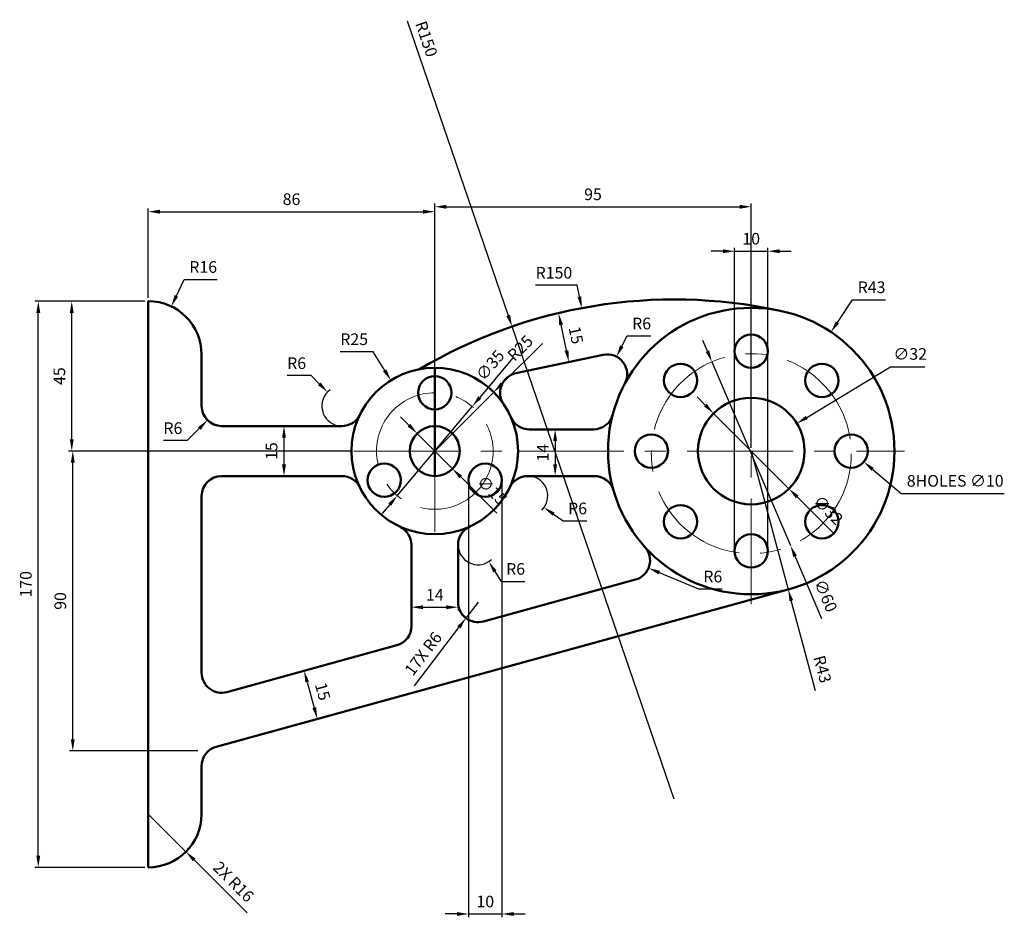
# Model space of a CAD drawing. Units: millimetres. Extents: x -39 to 257, y -15 to 255.
import ezdxf

# ---------------------------------------------------------------- set-up
doc = ezdxf.new("R2010")
doc.units = ezdxf.units.MM
doc.linetypes.add('CENTER', pattern=[50.8, 31.75, -6.35, 6.35, -6.35])
for name, color, linetype, lineweight in [('M-CNTR', 4, 'CENTER', 18), ('M-CONS', 8, 'Continuous', 13), ('M-DIMS', 3, 'Continuous', 25), ('M-OUTL', 7, 'Continuous', 50)]:
    doc.layers.add(name, color=color, linetype=linetype, lineweight=lineweight)
doc.styles.get("Standard").update_dxf_attribs({"font": 'arial.ttf'})
doc.dimstyles.new('AM_ISO$0', dxfattribs={"dimtxt": 3.5, "dimasz": 3.5, "dimexe": 1, "dimexo": 1, "dimgap": 1.5, "dimtad": 1, "dimdsep": 46, "dimtxsty": 'Standard', "dimcen": 0, "dimclrd": 256, "dimclre": 256, "dimclrt": 2, "dimadec": 0, "dimazin": 2, "dimtp": 0.1, "dimtm": 0.1, "dimtfac": 0.71, "dimtdec": 3, "dimtmove": 0, "dimatfit": 3, "dimfxl": 1, "dimlwd": -1, "dimlwe": -1, "dimarcsym": 1})
doc.dimstyles.new('AM_ISO$3', dxfattribs={"dimtxt": 3.5, "dimasz": 3.5, "dimexe": 1, "dimexo": 1, "dimgap": 1.5, "dimtad": 1, "dimtoh": 1, "dimdsep": 46, "dimtxsty": 'Standard', "dimcen": 0, "dimclrd": 256, "dimclre": 256, "dimclrt": 2, "dimadec": 0, "dimazin": 2, "dimtp": 0.1, "dimtm": 0.1, "dimtfac": 0.71, "dimtdec": 3, "dimtofl": 0, "dimtmove": 0, "dimatfit": 0, "dimfxl": 1, "dimlwd": -1, "dimlwe": -1, "dimarcsym": 1})
doc.dimstyles.new('AM_ISO$4', dxfattribs={"dimtxt": 3.5, "dimasz": 3.5, "dimexe": 1, "dimexo": 1, "dimgap": 1.5, "dimtad": 1, "dimtoh": 1, "dimdsep": 46, "dimtxsty": 'Standard', "dimcen": 0, "dimclrd": 256, "dimclre": 256, "dimclrt": 2, "dimadec": 0, "dimazin": 2, "dimtp": 0.1, "dimtm": 0.1, "dimtfac": 0.71, "dimtdec": 3, "dimtofl": 0, "dimtmove": 0, "dimatfit": 0, "dimfxl": 1, "dimlwd": -1, "dimlwe": -1, "dimarcsym": 1})

# ---------------------------------------------------------------- blocks, each defined once
blk = doc.blocks.new('*D3')
at = {"layer": 'Defpoints', "color": 0, "transparency": 16777216}
for p in [(-33.02, 170), (0, 170), (0, 0)]:
    blk.add_point(p, dxfattribs=at)
at = {"layer": 'M-DIMS', "color": 0, "linetype": 'ByBlock', "transparency": 16777216}
for p, q in [((-1, 170), (-34.02, 170)), ((-33.02, 3.5), (-33.02, 166.5)), ((-1, 0), (-34.02, 0))]:
    blk.add_line(p, q, dxfattribs=at)
at = {"layer": 'M-DIMS', "color": 0, "transparency": 16777216}
for points in [[(-33.61, 166.5), (-32.44, 166.5), (-33.02, 170)], [(-33.61, 3.5), (-32.44, 3.5), (-33.02, 0)]]:
    blk.add_solid(points, dxfattribs=at)
at = {"layer": 'M-DIMS', "color": 0, "transparency": 16777216, "insert": (-36.31, 85), "char_height": 3.5, "attachment_point": 5, "rotation": 90}
blk.add_mtext('170', dxfattribs=at)
blk = doc.blocks.new('*U4')
blk.add_circle((0, 0), 5)
blk = doc.blocks.new('*U5')
at = {"layer": 'M-OUTL', "color": 0, "linetype": 'ByBlock', "lineweight": -2, "transparency": 16777216}
for p, rotation in [((181, 154.99), 90), ((159.79, 146.21), 135), ((202.21, 146.21), 45), ((151.01, 125), 180), ((159.79, 103.79), 225), ((202.21, 103.79), 315), ((181, 95.01), 270)]:
    blk.add_blockref('*U4', p, dxfattribs=dict(at, rotation=rotation))
blk.add_blockref('*U4', (210.99, 125), dxfattribs=at)
blk = doc.blocks.new('*U6')
blk.add_circle((0, 0), 5)
blk = doc.blocks.new('*U7')
at = {"layer": 'M-OUTL', "color": 0, "linetype": 'ByBlock', "lineweight": -2, "transparency": 16777216}
blk.add_blockref('*U6', (86, 142.5), dxfattribs=at)
for p, rotation in [((70.84, 116.25), 120), ((101.16, 116.25), 240)]:
    blk.add_blockref('*U6', p, dxfattribs=dict(at, rotation=rotation))
blk = doc.blocks.new('*D8')
at = {"layer": 'Defpoints', "color": 0, "transparency": 16777216}
for p in [(144.62, 92.17), (150.16, 89.85)]:
    blk.add_point(p, dxfattribs=at)
at = {"layer": 'M-DIMS', "color": 0, "linetype": 'ByBlock', "transparency": 16777216}
for p, q in [((153.38, 88.5), (165.14, 83.58)), ((165.14, 83.58), (172.28, 83.58))]:
    blk.add_line(p, q, dxfattribs=at)
at = {"layer": 'M-DIMS', "color": 0, "transparency": 16777216}
blk.add_solid([(153.61, 89.04), (153.16, 87.96), (150.16, 89.85)], dxfattribs=at)
at = {"layer": 'M-DIMS', "color": 0, "transparency": 16777216, "insert": (169.46, 86.86), "char_height": 3.5, "attachment_point": 5}
blk.add_mtext('R6', dxfattribs=at)
blk = doc.blocks.new('*D9')
at = {"layer": 'Defpoints', "color": 0, "transparency": 16777216}
for p in [(99, 96.86), (102.2, 91.78)]:
    blk.add_point(p, dxfattribs=at)
at = {"layer": 'M-DIMS', "color": 0, "linetype": 'ByBlock', "transparency": 16777216}
for p, q in [((104.07, 88.83), (105.94, 85.87)), ((105.94, 85.87), (113.08, 85.87))]:
    blk.add_line(p, q, dxfattribs=at)
blk.add_arc((99, 96.86), 6, 189.5493, 311.8304, dxfattribs=at)
at = {"layer": 'M-DIMS', "color": 0, "transparency": 16777216}
blk.add_solid([(104.57, 89.14), (103.58, 88.51), (102.2, 91.78)], dxfattribs=at)
at = {"layer": 'M-DIMS', "color": 0, "transparency": 16777216, "insert": (110.26, 89.15), "char_height": 3.5, "attachment_point": 5}
blk.add_mtext('R6', dxfattribs=at)
blk = doc.blocks.new('*D10')
at = {"layer": 'Defpoints', "color": 0, "transparency": 16777216}
for p in [(22, 138.5), (17.77, 134.25)]:
    blk.add_point(p, dxfattribs=at)
at = {"layer": 'M-DIMS', "color": 0, "linetype": 'ByBlock', "transparency": 16777216}
for p, q in [((15.3, 131.76), (11.7, 128.14)), ((11.7, 128.14), (4.56, 128.14))]:
    blk.add_line(p, q, dxfattribs=at)
at = {"layer": 'M-DIMS', "color": 0, "transparency": 16777216}
blk.add_solid([(14.89, 132.17), (15.72, 131.35), (17.77, 134.25)], dxfattribs=at)
at = {"layer": 'M-DIMS', "color": 0, "transparency": 16777216, "insert": (7.38, 131.42), "char_height": 3.5, "attachment_point": 5}
blk.add_mtext('R6', dxfattribs=at)
blk = doc.blocks.new('*D11')
at = {"layer": 'Defpoints', "color": 0, "transparency": 16777216}
for p in [(86, 196.87), (0, 170), (86, 125)]:
    blk.add_point(p, dxfattribs=at)
at = {"layer": 'M-DIMS', "color": 0, "linetype": 'ByBlock', "transparency": 16777216}
for p, q in [((0, 171), (0, 197.87)), ((3.5, 196.87), (82.5, 196.87)), ((86, 126), (86, 197.87))]:
    blk.add_line(p, q, dxfattribs=at)
at = {"layer": 'M-DIMS', "color": 0, "transparency": 16777216}
for points in [[(3.5, 197.45), (3.5, 196.28), (0, 196.87)], [(82.5, 197.45), (82.5, 196.28), (86, 196.87)]]:
    blk.add_solid(points, dxfattribs=at)
at = {"layer": 'M-DIMS', "color": 0, "transparency": 16777216, "insert": (43, 200.16), "char_height": 3.5, "attachment_point": 5}
blk.add_mtext('86', dxfattribs=at)
blk = doc.blocks.new('*D12')
at = {"layer": 'Defpoints', "color": 0, "transparency": 16777216}
for p in [(181, 198.35), (86, 125), (181, 125)]:
    blk.add_point(p, dxfattribs=at)
at = {"layer": 'M-DIMS', "color": 0, "linetype": 'ByBlock', "transparency": 16777216}
for p, q in [((86, 126), (86, 199.35)), ((89.5, 198.35), (177.5, 198.35)), ((181, 126), (181, 199.35))]:
    blk.add_line(p, q, dxfattribs=at)
at = {"layer": 'M-DIMS', "color": 0, "transparency": 16777216}
for points in [[(89.5, 198.93), (89.5, 197.76), (86, 198.35)], [(177.5, 198.93), (177.5, 197.76), (181, 198.35)]]:
    blk.add_solid(points, dxfattribs=at)
at = {"layer": 'M-DIMS', "color": 0, "transparency": 16777216, "insert": (133.5, 201.63), "char_height": 3.5, "attachment_point": 5}
blk.add_mtext('95', dxfattribs=at)
blk = doc.blocks.new('*D13')
at = {"layer": 'Defpoints', "color": 0, "transparency": 16777216}
for p in [(6.91, 168.43), (0, 154)]:
    blk.add_point(p, dxfattribs=at)
at = {"layer": 'M-DIMS', "color": 0, "linetype": 'ByBlock', "transparency": 16777216}
for p, q in [((8.43, 171.59), (10.79, 176.52)), ((10.79, 176.52), (20.65, 176.52))]:
    blk.add_line(p, q, dxfattribs=at)
at = {"layer": 'M-DIMS', "color": 0, "transparency": 16777216}
blk.add_solid([(7.9, 171.84), (8.95, 171.33), (6.91, 168.43)], dxfattribs=at)
at = {"layer": 'M-DIMS', "color": 0, "transparency": 16777216, "insert": (16.47, 179.81), "char_height": 3.5, "attachment_point": 5}
blk.add_mtext('R16', dxfattribs=at)
blk = doc.blocks.new('*D14')
at = {"layer": 'Defpoints', "color": 0, "transparency": 16777216}
for p in [(49.09, 59.66), (50.75, 44.56), (53.07, 45.2)]:
    blk.add_point(p, dxfattribs=at)
at = {"layer": 'M-DIMS', "color": 0, "linetype": 'ByBlock', "transparency": 16777216}
for p, q in [((48.13, 59.4), (45.81, 58.76)), ((47.7, 55.65), (49.82, 47.94)), ((52.11, 44.94), (49.79, 44.3))]:
    blk.add_line(p, q, dxfattribs=at)
at = {"layer": 'M-DIMS', "color": 0, "transparency": 16777216}
for points in [[(48.26, 55.81), (47.14, 55.5), (46.77, 59.02)], [(50.39, 48.09), (49.26, 47.78), (50.75, 44.56)]]:
    blk.add_solid(points, dxfattribs=at)
at = {"layer": 'M-DIMS', "color": 0, "transparency": 16777216, "insert": (51.93, 52.67), "char_height": 3.5, "attachment_point": 5, "rotation": 285.3849}
blk.add_mtext('15', dxfattribs=at)
blk = doc.blocks.new('*D15')
at = {"layer": 'Defpoints', "color": 0, "transparency": 16777216}
for p in [(79, 84.66), (93, 84.66), (93, 78.11)]:
    blk.add_point(p, dxfattribs=at)
at = {"layer": 'M-DIMS', "color": 0, "linetype": 'ByBlock', "transparency": 16777216}
for p, q in [((79, 83.66), (79, 77.11)), ((93, 83.66), (93, 77.11)), ((82.5, 78.11), (89.5, 78.11))]:
    blk.add_line(p, q, dxfattribs=at)
at = {"layer": 'M-DIMS', "color": 0, "transparency": 16777216}
for points in [[(82.5, 78.69), (82.5, 77.52), (79, 78.11)], [(89.5, 78.69), (89.5, 77.52), (93, 78.11)]]:
    blk.add_solid(points, dxfattribs=at)
at = {"layer": 'M-DIMS', "color": 0, "transparency": 16777216, "insert": (86, 81.36), "char_height": 3.5, "attachment_point": 5}
blk.add_mtext('14', dxfattribs=at)
blk = doc.blocks.new('*D16')
at = {"layer": 'Defpoints', "color": 0, "transparency": 16777216}
for p in [(40.05, 132.5), (40.74, 132.5), (40.05, 117.5)]:
    blk.add_point(p, dxfattribs=at)
at = {"layer": 'M-DIMS', "color": 0, "linetype": 'ByBlock', "transparency": 16777216}
for p, q in [((41.05, 132.5), (41.74, 132.5)), ((40.74, 121), (40.74, 129)), ((41.05, 117.5), (41.74, 117.5))]:
    blk.add_line(p, q, dxfattribs=at)
at = {"layer": 'M-DIMS', "color": 0, "transparency": 16777216}
for points in [[(40.15, 129), (41.32, 129), (40.74, 132.5)], [(40.15, 121), (41.32, 121), (40.74, 117.5)]]:
    blk.add_solid(points, dxfattribs=at)
at = {"layer": 'M-DIMS', "color": 0, "transparency": 16777216, "insert": (37.45, 125), "char_height": 3.5, "attachment_point": 5, "rotation": 90}
blk.add_mtext('15', dxfattribs=at)
blk = doc.blocks.new('*D17')
at = {"layer": 'Defpoints', "color": 0, "transparency": 16777216}
for p in [(-22.67, 125), (62.15, 125), (15.85, 34.96)]:
    blk.add_point(p, dxfattribs=at)
at = {"layer": 'M-DIMS', "color": 0, "linetype": 'ByBlock', "transparency": 16777216}
for p, q in [((61.15, 125), (-23.67, 125)), ((-22.67, 38.46), (-22.67, 121.5)), ((14.85, 34.96), (-23.67, 34.96))]:
    blk.add_line(p, q, dxfattribs=at)
at = {"layer": 'M-DIMS', "color": 0, "transparency": 16777216}
for points in [[(-23.26, 121.5), (-22.09, 121.5), (-22.67, 125)], [(-23.26, 38.46), (-22.09, 38.46), (-22.67, 34.96)]]:
    blk.add_solid(points, dxfattribs=at)
at = {"layer": 'M-DIMS', "color": 0, "transparency": 16777216, "insert": (-25.96, 79.98), "char_height": 3.5, "attachment_point": 5, "rotation": 90}
blk.add_mtext('90', dxfattribs=at)
blk = doc.blocks.new('*D18')
at = {"layer": 'Defpoints', "color": 0, "transparency": 16777216}
for p in [(-22.97, 170), (0, 170), (61, 125)]:
    blk.add_point(p, dxfattribs=at)
at = {"layer": 'M-DIMS', "color": 0, "linetype": 'ByBlock', "transparency": 16777216}
for p, q in [((-1, 170), (-23.97, 170)), ((-22.97, 128.5), (-22.97, 166.5)), ((60, 125), (-23.97, 125))]:
    blk.add_line(p, q, dxfattribs=at)
at = {"layer": 'M-DIMS', "color": 0, "transparency": 16777216}
for points in [[(-23.56, 166.5), (-22.39, 166.5), (-22.97, 170)], [(-23.56, 128.5), (-22.39, 128.5), (-22.97, 125)]]:
    blk.add_solid(points, dxfattribs=at)
at = {"layer": 'M-DIMS', "color": 0, "transparency": 16777216, "insert": (-26.25, 147.5), "char_height": 3.5, "attachment_point": 5, "rotation": 90}
blk.add_mtext('45', dxfattribs=at)
blk = doc.blocks.new('*D19')
at = {"layer": 'Defpoints', "color": 0, "transparency": 16777216}
for p in [(53.83, 142.72), (58.09, 138.5)]:
    blk.add_point(p, dxfattribs=at)
at = {"layer": 'M-DIMS', "color": 0, "linetype": 'ByBlock', "transparency": 16777216}
for p, q in [((48.85, 147.64), (41.71, 147.64)), ((51.34, 145.18), (48.85, 147.64))]:
    blk.add_line(p, q, dxfattribs=at)
blk.add_arc((58.09, 138.5), 6, 125.7636, 260.4507, dxfattribs=at)
at = {"layer": 'M-DIMS', "color": 0, "transparency": 16777216}
blk.add_solid([(51.75, 145.6), (50.93, 144.77), (53.83, 142.72)], dxfattribs=at)
at = {"layer": 'M-DIMS', "color": 0, "transparency": 16777216, "insert": (44.53, 150.93), "char_height": 3.5, "attachment_point": 5}
blk.add_mtext('R6', dxfattribs=at)
blk = doc.blocks.new('*D20')
at = {"layer": 'Defpoints', "color": 0, "transparency": 16777216}
for p in [(204.93, 160.73), (181, 125)]:
    blk.add_point(p, dxfattribs=at)
at = {"layer": 'M-DIMS', "color": 0, "linetype": 'ByBlock', "transparency": 16777216}
for p, q in [((206.88, 163.63), (211.44, 170.44)), ((211.44, 170.44), (221.3, 170.44))]:
    blk.add_line(p, q, dxfattribs=at)
at = {"layer": 'M-DIMS', "color": 0, "transparency": 16777216}
blk.add_solid([(206.39, 163.96), (207.36, 163.31), (204.93, 160.73)], dxfattribs=at)
at = {"layer": 'M-DIMS', "color": 0, "transparency": 16777216, "insert": (217.12, 173.73), "char_height": 3.5, "attachment_point": 5}
blk.add_mtext('R43', dxfattribs=at)
blk = doc.blocks.new('*D21')
at = {"layer": 'Defpoints', "color": 0, "transparency": 16777216}
for p in [(72.82, 146.24), (86, 125)]:
    blk.add_point(p, dxfattribs=at)
at = {"layer": 'M-DIMS', "color": 0, "linetype": 'ByBlock', "transparency": 16777216}
for p, q in [((67.49, 154.83), (57.6, 154.83)), ((70.97, 149.22), (67.49, 154.83))]:
    blk.add_line(p, q, dxfattribs=at)
at = {"layer": 'M-DIMS', "color": 0, "transparency": 16777216}
blk.add_solid([(71.47, 149.52), (70.48, 148.91), (72.82, 146.24)], dxfattribs=at)
at = {"layer": 'M-DIMS', "color": 0, "transparency": 16777216, "insert": (61.8, 158.12), "char_height": 3.5, "attachment_point": 5}
blk.add_mtext('R25', dxfattribs=at)
blk = doc.blocks.new('*D22')
at = {"layer": 'Defpoints', "color": 0, "transparency": 16777216}
for p in [(119.62, 165.55), (123.19, 166.31), (123.43, 151.14)]:
    blk.add_point(p, dxfattribs=at)
at = {"layer": 'M-DIMS', "color": 0, "linetype": 'ByBlock', "transparency": 16777216}
for p, q in [((120.6, 165.76), (124.17, 166.51)), ((125.55, 155.16), (123.91, 162.88)), ((124.41, 151.34), (127.25, 151.94))]:
    blk.add_line(p, q, dxfattribs=at)
at = {"layer": 'M-DIMS', "color": 0, "transparency": 16777216}
for points in [[(124.48, 163), (123.34, 162.76), (123.19, 166.31)], [(126.12, 155.28), (124.97, 155.04), (126.27, 151.74)]]:
    blk.add_solid(points, dxfattribs=at)
at = {"layer": 'M-DIMS', "color": 0, "transparency": 16777216, "insert": (127.95, 159.7), "char_height": 3.5, "attachment_point": 5, "rotation": 281.9288}
blk.add_mtext('15', dxfattribs=at)
blk = doc.blocks.new('*D23')
at = {"layer": 'Defpoints', "color": 0, "transparency": 16777216}
for p in [(123.99, 131.5), (122.13, 117.5), (123.99, 117.5)]:
    blk.add_point(p, dxfattribs=at)
at = {"layer": 'M-DIMS', "color": 0, "linetype": 'ByBlock', "transparency": 16777216}
for p, q in [((122.99, 131.5), (121.13, 131.5)), ((122.13, 128), (122.13, 121)), ((122.99, 117.5), (121.13, 117.5))]:
    blk.add_line(p, q, dxfattribs=at)
at = {"layer": 'M-DIMS', "color": 0, "transparency": 16777216}
for points in [[(121.55, 128), (122.71, 128), (122.13, 131.5)], [(121.55, 121), (122.71, 121), (122.13, 117.5)]]:
    blk.add_solid(points, dxfattribs=at)
at = {"layer": 'M-DIMS', "color": 0, "transparency": 16777216, "insert": (118.87, 124.5), "char_height": 3.5, "attachment_point": 5, "rotation": 90}
blk.add_mtext('14', dxfattribs=at)
blk = doc.blocks.new('*D24')
at = {"layer": 'Defpoints', "color": 0, "transparency": 16777216}
for p in [(140.52, 153.35), (137.75, 148.03)]:
    blk.add_point(p, dxfattribs=at)
at = {"layer": 'M-DIMS', "color": 0, "linetype": 'ByBlock', "transparency": 16777216}
for p, q in [((142.14, 156.45), (143.76, 159.56)), ((143.76, 159.56), (150.9, 159.56))]:
    blk.add_line(p, q, dxfattribs=at)
at = {"layer": 'M-DIMS', "color": 0, "transparency": 16777216}
blk.add_solid([(141.62, 156.72), (142.66, 156.18), (140.52, 153.35)], dxfattribs=at)
at = {"layer": 'M-DIMS', "color": 0, "transparency": 16777216, "insert": (148.08, 162.84), "char_height": 3.5, "attachment_point": 5}
blk.add_mtext('R6', dxfattribs=at)
blk = doc.blocks.new('*D25')
at = {"layer": 'Defpoints', "color": 0, "transparency": 16777216}
for p in [(113.91, 111.5), (118.81, 108.05)]:
    blk.add_point(p, dxfattribs=at)
at = {"layer": 'M-DIMS', "color": 0, "linetype": 'ByBlock', "transparency": 16777216}
for p, q in [((121.68, 106.03), (124.54, 104.02)), ((124.54, 104.02), (131.68, 104.02))]:
    blk.add_line(p, q, dxfattribs=at)
blk.add_arc((113.91, 111.5), 6, 315.3211, 80.4507, dxfattribs=at)
at = {"layer": 'M-DIMS', "color": 0, "transparency": 16777216}
blk.add_solid([(122.01, 106.51), (121.34, 105.56), (118.81, 108.05)], dxfattribs=at)
at = {"layer": 'M-DIMS', "color": 0, "transparency": 16777216, "insert": (128.86, 107.31), "char_height": 3.5, "attachment_point": 5}
blk.add_mtext('R6', dxfattribs=at)
blk = doc.blocks.new('*D26')
at = {"layer": 'Defpoints', "color": 0, "transparency": 16777216}
for p in [(194.69, 133.29), (167.31, 116.71)]:
    blk.add_point(p, dxfattribs=at)
at = {"layer": 'M-DIMS', "color": 0, "linetype": 'ByBlock', "transparency": 16777216}
for p, q in [((197.68, 135.1), (222.83, 150.32)), ((222.83, 150.32), (233.11, 150.32))]:
    blk.add_line(p, q, dxfattribs=at)
at = {"layer": 'M-DIMS', "color": 0, "transparency": 16777216}
blk.add_solid([(197.38, 135.6), (197.98, 134.6), (194.69, 133.29)], dxfattribs=at)
at = {"layer": 'M-DIMS', "color": 0, "transparency": 16777216, "insert": (228.72, 153.7), "char_height": 3.5, "attachment_point": 5}
blk.add_mtext('∅32', dxfattribs=at)
blk = doc.blocks.new('*D27')
at = {"layer": 'Defpoints', "color": 0, "transparency": 16777216}
for p in [(207.18, 128.24), (214.8, 121.76)]:
    blk.add_point(p, dxfattribs=at)
at = {"layer": 'M-DIMS', "color": 0, "linetype": 'ByBlock', "transparency": 16777216}
for p, q in [((217.46, 119.49), (226, 112.22)), ((226, 112.22), (256.96, 112.22))]:
    blk.add_line(p, q, dxfattribs=at)
at = {"layer": 'M-DIMS', "color": 0, "transparency": 16777216}
blk.add_solid([(217.84, 119.93), (217.08, 119.05), (214.8, 121.76)], dxfattribs=at)
at = {"layer": 'M-DIMS', "color": 0, "transparency": 16777216, "insert": (242.23, 115.6), "char_height": 3.5, "attachment_point": 5}
blk.add_mtext('8HOLES ∅10', dxfattribs=at)
blk = doc.blocks.new('*D28')
at = {"layer": 'Defpoints', "color": 0, "transparency": 16777216}
for p in [(130.09, 167.92), (157.88, 20.52)]:
    blk.add_point(p, dxfattribs=at)
at = {"layer": 'M-DIMS', "color": 0, "linetype": 'ByBlock', "transparency": 16777216}
for p, q in [((128.79, 174.8), (116.22, 174.8)), ((129.44, 171.36), (128.79, 174.8))]:
    blk.add_line(p, q, dxfattribs=at)
at = {"layer": 'M-DIMS', "color": 0, "transparency": 16777216}
blk.add_solid([(130.01, 171.47), (128.87, 171.25), (130.09, 167.92)], dxfattribs=at)
at = {"layer": 'M-DIMS', "color": 0, "transparency": 16777216, "insert": (121.76, 178.08), "char_height": 3.5, "attachment_point": 5}
blk.add_mtext('R150', dxfattribs=at)
blk = doc.blocks.new('*D29')
at = {"layer": 'Defpoints', "color": 0, "transparency": 16777216}
for p in [(186, 185), (176, 95.01), (186, 95.01)]:
    blk.add_point(p, dxfattribs=at)
at = {"layer": 'M-DIMS', "linetype": 'ByBlock', "transparency": 16777216}
for p, q in [((172.5, 185), (169, 185)), ((176, 96.01), (176, 186)), ((176, 185), (186, 185)), ((186, 96.01), (186, 186)), ((189.5, 185), (193, 185))]:
    blk.add_line(p, q, dxfattribs=at)
at = {"layer": 'M-DIMS', "transparency": 16777216}
for points in [[(172.5, 185.58), (172.5, 184.42), (176, 185)], [(189.5, 185.58), (189.5, 184.42), (186, 185)]]:
    blk.add_solid(points, dxfattribs=at)
at = {"layer": 'M-DIMS', "color": 2, "transparency": 16777216, "insert": (181, 188.29), "char_height": 3.5, "attachment_point": 5}
blk.add_mtext('10', dxfattribs=at)
blk = doc.blocks.new('*D30')
at = {"layer": 'Defpoints', "color": 0, "transparency": 16777216}
for p in [(96.16, 116.25), (106.16, 116.25), (106.16, -14)]:
    blk.add_point(p, dxfattribs=at)
at = {"layer": 'M-DIMS', "linetype": 'ByBlock', "transparency": 16777216}
for p, q in [((96.16, 115.25), (96.16, -15)), ((106.16, 115.25), (106.16, -15)), ((92.66, -14), (89.16, -14)), ((96.16, -14), (106.16, -14)), ((109.66, -14), (113.16, -14))]:
    blk.add_line(p, q, dxfattribs=at)
at = {"layer": 'M-DIMS', "transparency": 16777216}
for points in [[(92.66, -13.42), (92.66, -14.58), (96.16, -14)], [(109.66, -13.42), (109.66, -14.58), (106.16, -14)]]:
    blk.add_solid(points, dxfattribs=at)
at = {"layer": 'M-DIMS', "color": 2, "transparency": 16777216, "insert": (101.16, -10.71), "char_height": 3.5, "attachment_point": 5}
blk.add_mtext('10', dxfattribs=at)
blk = doc.blocks.new('*D31')
at = {"layer": 'Defpoints', "color": 0, "transparency": 16777216}
for p in [(109.18, 162.39), (157.88, 20.52)]:
    blk.add_point(p, dxfattribs=at)
at = {"layer": 'M-DIMS', "linetype": 'ByBlock', "transparency": 16777216}
for p, q in [((77.67, 254.17), (108.04, 165.7)), ((157.88, 20.52), (109.18, 162.39))]:
    blk.add_line(p, q, dxfattribs=at)
at = {"layer": 'M-DIMS', "transparency": 16777216}
blk.add_solid([(108.6, 165.89), (107.49, 165.51), (109.18, 162.39)], dxfattribs=at)
at = {"layer": 'M-DIMS', "color": 2, "transparency": 16777216, "insert": (83.07, 248.58), "char_height": 3.5, "attachment_point": 5, "rotation": 288.9467}
blk.add_mtext('R150', dxfattribs=at)
blk = doc.blocks.new('*D32')
at = {"layer": 'Defpoints', "color": 0, "transparency": 16777216}
for p in [(181, 125), (192.11, 83.46)]:
    blk.add_point(p, dxfattribs=at)
at = {"layer": 'M-DIMS', "linetype": 'ByBlock', "transparency": 16777216}
for p, q in [((181, 125), (192.11, 83.46)), ((200.25, 53.05), (193.01, 80.08))]:
    blk.add_line(p, q, dxfattribs=at)
at = {"layer": 'M-DIMS', "transparency": 16777216}
blk.add_solid([(193.58, 80.23), (192.45, 79.93), (192.11, 83.46)], dxfattribs=at)
at = {"layer": 'M-DIMS', "color": 2, "transparency": 16777216, "insert": (201.95, 59.39), "char_height": 3.5, "attachment_point": 5, "rotation": 284.9744}
blk.add_mtext('R43', dxfattribs=at)
blk = doc.blocks.new('*D33')
at = {"layer": 'Defpoints', "color": 0, "transparency": 16777216}
for p in [(103.68, 142.68), (86, 125)]:
    blk.add_point(p, dxfattribs=at)
at = {"layer": 'M-DIMS', "linetype": 'ByBlock', "transparency": 16777216}
for p, q in [((118.31, 157.31), (106.15, 145.15)), ((86, 125), (103.68, 142.68))]:
    blk.add_line(p, q, dxfattribs=at)
at = {"layer": 'M-DIMS', "transparency": 16777216}
blk.add_solid([(105.74, 145.57), (106.57, 144.74), (103.68, 142.68)], dxfattribs=at)
at = {"layer": 'M-DIMS', "color": 2, "transparency": 16777216, "insert": (111.96, 155.61), "char_height": 3.5, "attachment_point": 5, "rotation": 45}
blk.add_mtext('R25', dxfattribs=at)
blk = doc.blocks.new('*D34')
at = {"layer": 'Defpoints', "color": 0, "transparency": 16777216}
for p in [(0, 16), (11.31, 4.69)]:
    blk.add_point(p, dxfattribs=at)
at = {"layer": 'M-DIMS', "linetype": 'ByBlock', "transparency": 16777216}
for p, q in [((0, 16), (11.31, 4.69)), ((29.66, -13.66), (13.79, 2.21))]:
    blk.add_line(p, q, dxfattribs=at)
at = {"layer": 'M-DIMS', "transparency": 16777216}
blk.add_solid([(14.2, 2.62), (13.38, 1.8), (11.31, 4.69)], dxfattribs=at)
at = {"layer": 'M-DIMS', "color": 2, "transparency": 16777216, "insert": (25.28, -4.64), "char_height": 3.5, "attachment_point": 5, "rotation": 315}
blk.add_mtext('2X R16', dxfattribs=at)
blk = doc.blocks.new('*D35')
at = {"layer": 'Defpoints', "color": 0, "transparency": 16777216}
for p in [(99, 79.62), (95.36, 74.85)]:
    blk.add_point(p, dxfattribs=at)
at = {"layer": 'M-DIMS', "linetype": 'ByBlock', "transparency": 16777216}
for p, q in [((99, 79.62), (95.36, 74.85)), ((79.87, 54.52), (93.24, 72.06))]:
    blk.add_line(p, q, dxfattribs=at)
at = {"layer": 'M-DIMS', "transparency": 16777216}
blk.add_solid([(92.78, 72.42), (93.71, 71.71), (95.36, 74.85)], dxfattribs=at)
at = {"layer": 'M-DIMS', "color": 2, "transparency": 16777216, "insert": (82.88, 63.89), "char_height": 3.5, "attachment_point": 5, "rotation": 52.687}
blk.add_mtext('17X R6', dxfattribs=at)
blk = doc.blocks.new('*D36')
at = {"layer": 'Defpoints', "color": 0, "transparency": 16777216}
for p in [(169.69, 136.31), (192.31, 113.69)]:
    blk.add_point(p, dxfattribs=at)
at = {"layer": 'M-DIMS', "linetype": 'ByBlock', "transparency": 16777216}
for p, q in [((167.21, 138.79), (164.74, 141.26)), ((169.69, 136.31), (192.31, 113.69)), ((205.6, 100.4), (194.79, 111.21))]:
    blk.add_line(p, q, dxfattribs=at)
at = {"layer": 'M-DIMS', "transparency": 16777216}
for points in [[(167.62, 139.2), (166.8, 138.38), (169.69, 136.31)], [(195.2, 111.62), (194.38, 110.8), (192.31, 113.69)]]:
    blk.add_solid(points, dxfattribs=at)
at = {"layer": 'M-DIMS', "color": 2, "transparency": 16777216, "insert": (203.82, 106.96), "char_height": 3.5, "attachment_point": 5, "rotation": 315}
blk.add_mtext('∅32', dxfattribs=at)
blk = doc.blocks.new('*D37')
at = {"layer": 'Defpoints', "color": 0, "transparency": 16777216}
for p in [(80.7, 130.3), (91.3, 119.7)]:
    blk.add_point(p, dxfattribs=at)
at = {"layer": 'M-DIMS', "linetype": 'ByBlock', "transparency": 16777216}
for p, q in [((78.22, 132.78), (75.75, 135.25)), ((80.7, 130.3), (91.3, 119.7)), ((104.63, 106.37), (93.78, 117.22))]:
    blk.add_line(p, q, dxfattribs=at)
at = {"layer": 'M-DIMS', "transparency": 16777216}
for points in [[(78.63, 133.19), (77.81, 132.37), (80.7, 130.3)], [(94.19, 117.63), (93.37, 116.81), (91.3, 119.7)]]:
    blk.add_solid(points, dxfattribs=at)
at = {"layer": 'M-DIMS', "color": 2, "transparency": 16777216, "insert": (102.84, 112.95), "char_height": 3.5, "attachment_point": 5, "rotation": 315}
blk.add_mtext('∅15', dxfattribs=at)
blk = doc.blocks.new('*D38')
at = {"layer": 'Defpoints', "color": 0, "transparency": 16777216}
for p in [(97.25, 138.4), (74.75, 111.6)]:
    blk.add_point(p, dxfattribs=at)
at = {"layer": 'M-DIMS', "linetype": 'ByBlock', "transparency": 16777216}
for p, q in [((109.37, 152.84), (99.5, 141.08)), ((74.75, 111.6), (97.25, 138.4)), ((72.5, 108.92), (70.25, 106.24))]:
    blk.add_line(p, q, dxfattribs=at)
at = {"layer": 'M-DIMS', "transparency": 16777216}
for points in [[(99.06, 141.46), (99.95, 140.71), (97.25, 138.4)], [(72.05, 109.29), (72.94, 108.54), (74.75, 111.6)]]:
    blk.add_solid(points, dxfattribs=at)
at = {"layer": 'M-DIMS', "color": 2, "transparency": 16777216, "insert": (102.97, 150.48), "char_height": 3.5, "attachment_point": 5, "rotation": 49.9848}
blk.add_mtext('∅35', dxfattribs=at)
blk = doc.blocks.new('*D39')
at = {"layer": 'Defpoints', "color": 0, "transparency": 16777216}
for p in [(169.21, 151.79), (192.79, 96.62)]:
    blk.add_point(p, dxfattribs=at)
at = {"layer": 'M-DIMS', "linetype": 'ByBlock', "transparency": 16777216}
for p, q in [((167.83, 155), (166.46, 158.22)), ((169.21, 151.79), (192.79, 96.62)), ((202.19, 74.64), (194.17, 93.4))]:
    blk.add_line(p, q, dxfattribs=at)
at = {"layer": 'M-DIMS', "transparency": 16777216}
for points in [[(168.37, 155.23), (167.3, 154.77), (169.21, 151.79)], [(194.7, 93.63), (193.63, 93.17), (192.79, 96.62)]]:
    blk.add_solid(points, dxfattribs=at)
at = {"layer": 'M-DIMS', "color": 2, "transparency": 16777216, "insert": (202.98, 81.4), "char_height": 3.5, "attachment_point": 5, "rotation": 293.1465}
blk.add_mtext('∅60', dxfattribs=at)

msp = doc.modelspace()

# ---------------------------------------------------------------- linework, layer by layer
at = {"layer": 'M-CNTR'}
for p, q in [((181, 79), (181, 171)), ((86, 100.694), (86, 149.306)), ((61.694, 125), (110.306, 125)), ((111, 125), (227, 125))]:
    msp.add_line(p, q, dxfattribs=at)
for centre, radius in [((181, 124.201), 30), ((86, 125), 17.5)]:
    msp.add_circle(centre, radius, dxfattribs=at)
at = {"layer": 'M-CONS'}
for p, q in [((0, 154), (0, 154)), ((245.959, 35), (245.959, 35)), ((0, 16), (0, 16)), ((0, 16), (0, 16))]:
    msp.add_line(p, q, dxfattribs=at)
at = {"layer": 'M-OUTL'}
for p, q in [((0, 0), (0, 170)), ((16, 138.5), (16, 154)), ((110.346, 148.373), (136.509, 153.901)), ((86, 117.5), (86, 150)), ((22, 132.5), (58.094, 132.5)), ((114.368, 131.5), (133.621, 131.5)), ((22, 117.5), (58.094, 117.5)), ((113.906, 117.5), (133.896, 117.5)), ((16, 58.431), (16, 111.5)), ((79, 72.465), (79, 96.858)), ((93, 79.619), (93, 96.858)), ((100.592, 73.834), (146.214, 86.387)), ((20.408, 36.213), (192.408, 83.541)), ((23.592, 52.646), (74.592, 66.68)), ((16, 16), (16, 30.428)), ((0, 16), (0, 20.9)), ((0, 0), (0, 16))]:
    msp.add_line(p, q, dxfattribs=at)
for centre, radius in [((181, 125), 43), ((86, 125), 25), ((181, 125), 16), ((86, 125), 7.5)]:
    msp.add_circle(centre, radius, dxfattribs=at)
for centre, radius, start, end in [((0, 154), 16, 0, 90), ((157.883, 20.516), 150, 77.96123, 120.63326), ((137.749, 148.03), 6, 331.96552, 101.9288), ((111.586, 142.503), 6, 101.9288, 214.37524), ((22, 138.5), 6, 180, 270), ((133.621, 137.5), 6, 270, 345.22037), ((58.094, 138.5), 6, 270, 334.18391), ((114.368, 137.5), 6, 203.77999, 270), ((22, 111.5), 6, 90, 180), ((58.094, 111.5), 6, 25.81609, 90), ((113.906, 111.5), 6, 90, 154.18391), ((133.896, 111.5), 6, 15.99242, 90), ((73, 96.858), 6, 0, 65.20614), ((99, 96.858), 6, 114.79386, 180), ((144.622, 92.172), 6, 285.38491, 42.06315), ((99, 79.619), 6, 180, 285.38491), ((73, 72.465), 6, 285.38491, 0), ((22, 58.431), 6, 180, 285.38491), ((22, 30.428), 6, 105.38491, 180), ((0, 16), 16, 270, 0)]:
    msp.add_arc(centre, radius, start, end, dxfattribs=at)

# ---------------------------------------------------------------- block references
for name in ['*U5', '*U7']:
    msp.add_blockref(name, (0, 0), dxfattribs=at)

# ---------------------------------------------------------------- dimensions: what is measured, and where the dimension line sits
at = {"layer": 'M-DIMS'}
for center, mpoint, dimstyle, override, picture, middle in [((157.883, 20.516), (109.18, 162.389), 'AM_ISO$0', {"dimdec": 0, "dimlfac": 1, "dimrnd": 0, "dimzin": 0, "dimdsep": 46, "dimlunit": 2}, '*D31', (79.958, 247.513)), ((0, 154), (6.914, 168.429), 'AM_ISO$4', {"dimpost": '', "dimclrd": 0, "dimclre": 0, "dimclrt": 0}, '*D13', (16.471, 176.52)), ((157.883, 20.516), (130.088, 167.918), 'AM_ISO$4', {"dimpost": '', "dimclrd": 0, "dimclre": 0, "dimclrt": 0}, '*D28', (121.755, 174.797)), ((181, 125), (204.932, 160.725), 'AM_ISO$4', {"dimpost": '', "dimclrd": 0, "dimclre": 0, "dimclrt": 0}, '*D20', (217.12, 170.439)), ((137.749, 148.03), (140.524, 153.35), 'AM_ISO$4', {"dimpost": '', "dimclrd": 0, "dimclre": 0, "dimclrt": 0}, '*D24', (148.081, 159.557)), ((86, 125), (72.819, 146.243), 'AM_ISO$4', {"dimclrd": 0, "dimclre": 0, "dimclrt": 0}, '*D21', (61.797, 154.829)), ((86, 125), (103.678, 142.678), 'AM_ISO$0', {"dimdec": 0, "dimlfac": 1, "dimrnd": 0, "dimzin": 0, "dimdsep": 46, "dimlunit": 2}, '*D33', (114.284, 153.284)), ((58.094, 138.5), (53.828, 142.719), 'AM_ISO$4', {"dimclrd": 0, "dimclre": 0, "dimclrt": 0}, '*D19', (44.531, 147.642)), ((22, 138.5), (17.769, 134.245), 'AM_ISO$4', {"dimpost": '', "dimclrd": 0, "dimclre": 0, "dimclrt": 0}, '*D10', (7.376, 128.138)), ((181, 125), (192.111, 83.46), 'AM_ISO$0', {"dimdec": 0, "dimlfac": 1, "dimrnd": 0, "dimzin": 0, "dimdsep": 46, "dimlunit": 2}, '*D32', (198.777, 58.536)), ((113.906, 111.5), (118.813, 108.047), 'AM_ISO$4', {"dimpost": '', "dimclrd": 0, "dimclre": 0, "dimclrt": 0}, '*D25', (128.859, 104.019)), ((99, 96.858), (102.204, 91.785), 'AM_ISO$4', {"dimpost": '', "dimclrd": 0, "dimclre": 0, "dimclrt": 0}, '*D9', (110.264, 85.867)), ((144.622, 92.172), (150.156, 89.854), 'AM_ISO$4', {"dimpost": '', "dimclrd": 0, "dimclre": 0, "dimclrt": 0}, '*D8', (169.462, 83.577))]:
    dim = msp.add_radius_dim(center=center, mpoint=mpoint, dimstyle=dimstyle, override=override, dxfattribs=at)
    dim.commit()
    dim.dimension.update_dxf_attribs({"geometry": picture, "text_midpoint": middle, "dimtype": 164})
for base, p1, p2, override, picture, middle in [((86, 196.868), (0, 170), (86, 125), {"dimpost": '', "dimclrd": 0, "dimclre": 0, "dimclrt": 0}, '*D11', (43, 200.155)), ((186, 185), (176, 95.011), (186, 95.011), {"dimdec": 0, "dimlfac": 1, "dimrnd": 0, "dimzin": 0, "dimdsep": 46, "dimlunit": 2}, '*D29', (181, 188.287)), ((106.155, -14), (96.155, 116.25), (106.155, 116.25), {"dimdec": 0, "dimlfac": 1, "dimrnd": 0, "dimzin": 0, "dimdsep": 46, "dimlunit": 2}, '*D30', (101.155, -10.713))]:
    dim = msp.add_linear_dim(base=base, p1=p1, p2=p2, dimstyle='AM_ISO$0', override=override, dxfattribs=at)
    dim.commit()
    dim.dimension.update_dxf_attribs({"geometry": picture, "text_midpoint": middle})
for base, p1, p2, angle, override, picture, middle in [((181, 198.348), (86, 125), (181, 125), 0, {"dimclrd": 0, "dimclre": 0, "dimclrt": 0}, '*D12', (133.5, 201.635)), ((-33.022, 170), (0, 0), (0, 170), 90, {"dimpost": '', "dimclrd": 0, "dimclre": 0, "dimclrt": 0}, '*D3', (-36.309, 85)), ((-22.973, 170), (61, 125), (0, 170), 90, {"dimpost": '', "dimclrd": 0, "dimclre": 0, "dimclrt": 0}, '*D18', (-26.253, 147.5)), ((123.191, 166.308), (123.428, 151.137), (119.624, 165.555), 101.9288, {"dimdec": 0, "dimclrd": 0, "dimclre": 0, "dimclrt": 0}, '*D22', (127.946, 159.702)), ((122.131, 117.5), (123.995, 131.5), (123.995, 117.5), 90, {"dimpost": '', "dimclrd": 0, "dimclre": 0, "dimclrt": 0}, '*D23', (118.874, 124.5)), ((-22.673, 125), (15.846, 34.958), (62.152, 125), 90, {"dimdec": 0, "dimclrd": 0, "dimclre": 0, "dimclrt": 0}, '*D17', (-25.96, 79.979))]:
    dim = msp.add_linear_dim(base=base, p1=p1, p2=p2, angle=angle, dimstyle='AM_ISO$0', override=override, dxfattribs=at)
    dim.commit()
    dim.dimension.update_dxf_attribs({"geometry": picture, "text_midpoint": middle})
for p1, p2, dimstyle, override, picture, middle in [((169.208, 151.786), (192.792, 96.616), 'AM_ISO$0', {"dimdec": 0, "dimlfac": 1, "dimrnd": 0, "dimzin": 0, "dimdsep": 46, "dimlunit": 2}, '*D39', (199.868, 80.065)), ((167.312, 116.714), (194.688, 133.286), 'AM_ISO$3', {"dimpost": '', "dimclrd": 0, "dimclre": 0, "dimclrt": 0}, '*D26', (228.719, 150.319)), ((169.686, 136.314), (192.314, 113.686), 'AM_ISO$0', {"dimdec": 0, "dimlfac": 1, "dimrnd": 0, "dimzin": 0, "dimdsep": 46, "dimlunit": 2}, '*D36', (201.43, 104.57))]:
    dim = msp.add_diameter_dim_2p(p1=p1, p2=p2, dimstyle=dimstyle, override=override, dxfattribs=at)
    dim.commit()
    dim.dimension.update_dxf_attribs({"geometry": picture, "text_midpoint": middle, "dimtype": 163})
for p1, p2, picture, middle in [((74.748, 111.597), (97.252, 138.403), '*D38', (105.562, 148.301)), ((80.697, 130.303), (91.303, 119.697), '*D37', (100.442, 110.558))]:
    dim = msp.add_diameter_dim_2p(p1=p1, p2=p2, dimstyle='AM_ISO$0', override={"dimdec": 0, "dimlfac": 1, "dimrnd": 0, "dimzin": 0, "dimdsep": 46, "dimlunit": 2}, dxfattribs=at)
    dim.commit()
    dim.dimension.update_dxf_attribs({"geometry": picture, "text_midpoint": middle})
for p1, p2, distance, override, picture, middle in [((40.047, 117.5), (40.047, 132.5), -0.688, {"dimclrd": 0, "dimclre": 0, "dimclrt": 0}, '*D16', (37.448, 125)), ((79, 84.661), (93, 84.661), -6.554, {"dimclrd": 0, "dimclre": 0, "dimclrt": 0}, '*D15', (86, 81.364)), ((49.092, 59.663), (53.071, 45.201), -2.406, {"dimpost": '', "dimclrd": 0, "dimclre": 0, "dimclrt": 0}, '*D14', (51.931, 52.666))]:
    dim = msp.add_aligned_dim(p1=p1, p2=p2, distance=distance, dimstyle='AM_ISO$0', override=override, dxfattribs=at)
    dim.commit()
    dim.dimension.update_dxf_attribs({"geometry": picture, "text_midpoint": middle})
dim = msp.add_diameter_dim_2p(p1=(207.182, 128.241), p2=(214.796, 121.759), text='8HOLES <>', dimstyle='AM_ISO$3', override={"dimpost": '', "dimclrd": 0, "dimclre": 0, "dimclrt": 0}, dxfattribs=at)
dim.commit()
dim.dimension.update_dxf_attribs({"geometry": '*D27', "text_midpoint": (242.233, 112.219), "dimtype": 163})
for center, mpoint, text, picture, middle in [((99, 79.619), (95.363, 74.847), '17X <>', '*D35', (82.883, 63.895)), ((0, 16), (11.314, 4.686), '2X <>', '*D34', (25.284, -4.636))]:
    dim = msp.add_radius_dim(center=center, mpoint=mpoint, text=text, dimstyle='AM_ISO$0', override={"dimdec": 0, "dimlfac": 1, "dimrnd": 0, "dimzin": 0, "dimdsep": 46, "dimlunit": 2}, dxfattribs=at)
    dim.commit()
    dim.dimension.update_dxf_attribs({"geometry": picture, "text_midpoint": middle})

doc.saveas('drawing.dxf')
